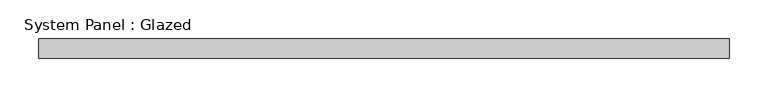
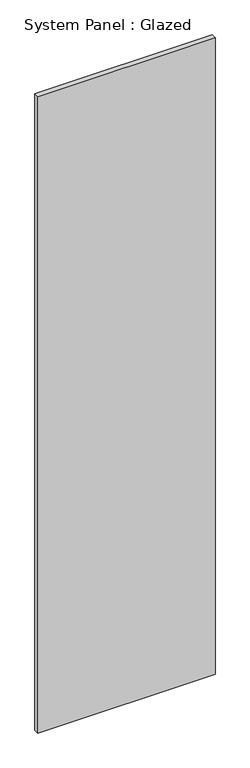
"""IFC4 building model written with IfcOpenShell, lengths in millimetres: plate geometry, System Panel : Glazed."""

from ifc_helpers import new_model, si_unit, origin, origin_with_axes, place, context, project, spatial, polyline, outline, extrude, source, transform, mapped, element, save


def system_panel_glazed_b03b416e(model_context):
    return source(origin(), model_context, "Body", "SweptSolid", [
        extrude(outline(polyline([(445.075, 19.05), (-445.075, 19.05), (-445.075, 44.45), (445.075, 44.45), (445.075, 19.05)])), origin_with_axes(), (0.0, 0.0, 1.0), 3379.9820397),
    ])


if __name__ == "__main__":
    model = new_model("IFC4")
    model_context = context("Model", 3, world=origin())
    ifc_project = project(units=[si_unit("LENGTHUNIT", "METRE", prefix="MILLI")], contexts=[model_context])
    site = spatial("IfcSite", under=ifc_project)
    building = spatial("IfcBuilding", under=site)
    placement = place(None, origin())
    system_panel_glazed_shape = system_panel_glazed_b03b416e(model_context)
    element("IfcPlate", 1, ObjectType="System Panel : Glazed", at=placement, inside=building, context=model_context, shape_type="MappedRepresentation", body=[
        mapped(system_panel_glazed_shape, transform((0.0, 0.0, 0.0), x_axis=(1.0, 0.0, 0.0), y_axis=(0.0, 1.0, 0.0), z_axis=(0.0, 0.0, 1.0))),
    ])
    save(model, "model.ifc")

# Revit data of these elements
# Type "System Panel : Glazed"
#   Construction Type Id = "GSP4R"
#   Analytic Construction = "1/8 in Pilkington single glazing"
#   Visual Light Transmittance = 0.9
#   Solar Heat Gain Coefficient = 0.86
#   Heat Transfer Coefficient (U) = 1.18115 BTU/(h·ft²·°F)
#   Define Thermal Properties by = 1
# Element 1 (IfcPlate, "System Panel : Glazed")
#   Materials on its faces: "Glass"
# Materials
#   "Glass": class "Glass", colour RGB 0 128 192, transparency 0.75, Description = "Soda Lime Glass", Cost = 0
